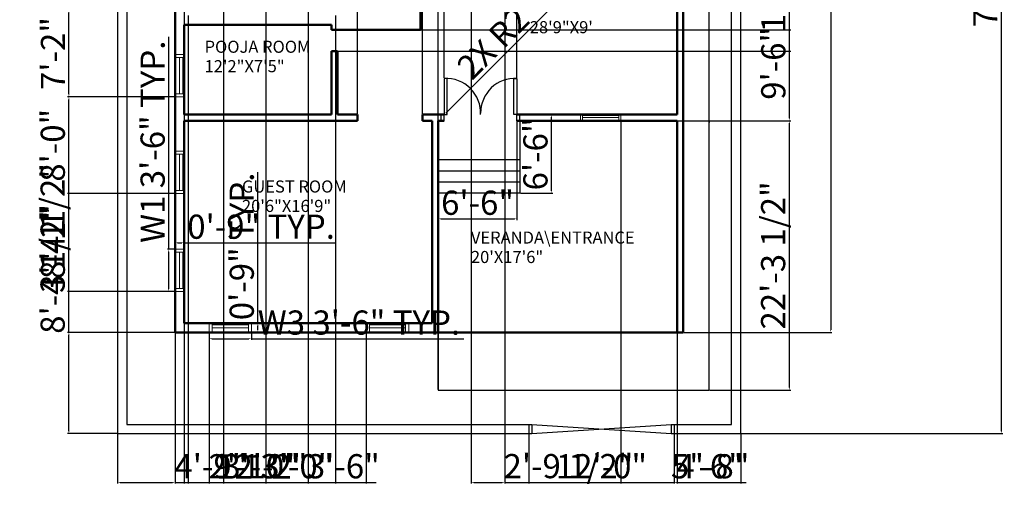
# Model space of a CAD drawing. Units: inches. Extents: x 2047 to 3023, y 479 to 1545.
# Tile 1 of 3: x 2047 to 3023, y 479 to 961. Entities that reach past the tile are written whole.
import ezdxf

# ---------------------------------------------------------------- set-up
doc = ezdxf.new("R2010")
doc.units = ezdxf.units.IN
for name, color, linetype, lineweight in [('A-ANNO-DIMS', 2, 'Continuous', 18), ('A-AREA-IDEN', 7, 'Continuous', 25), ('A-DOOR', 3, 'Continuous', 25), ('A-FLOR', 8, 'Continuous', 25), ('A-FLOR-STRS', 7, 'Continuous', 25), ('A-GLAZ', 4, 'Continuous', 18), ('A-WALL', 7, 'Continuous', 50), ('C-PROP', 8, 'Continuous', 30)]:
    doc.layers.add(name, color=color, linetype=linetype, lineweight=lineweight)
doc.styles.get("Standard").update_dxf_attribs({"font": 'arial.ttf'})
doc.dimstyles.new('ISO-25', dxfattribs={"dimtxt": 24, "dimasz": 2.5, "dimexe": 1.25, "dimexo": 0.625, "dimtad": 1, "dimdec": 1, "dimlunit": 3, "dimtxsty": 'Standard', "dimcen": 2.5, "dimadec": 0, "dimazin": 0, "dimtfac": 1, "dimtdec": 1, "dimtmove": 0, "dimatfit": 3, "dimfxl": 1, "dimarcsym": 0})

# ---------------------------------------------------------------- blocks, each defined once
blk = doc.blocks.new('*D3')
at = {"layer": 'A-ANNO-DIMS', "color": 0, "lineweight": -2, "transparency": 16777216}
for p, q in [((2762.53, 1447.48), (3021.8, 1447.48)), ((3020.55, 552.98), (3020.55, 1444.98)), ((2762.53, 550.48), (3021.8, 550.48))]:
    blk.add_line(p, q, dxfattribs=at)
at = {"layer": 'A-ANNO-DIMS', "color": 0, "transparency": 16777216}
for points in [[(3020.13, 1444.98), (3020.96, 1444.98), (3020.55, 1447.48)], [(3020.13, 552.98), (3020.96, 552.98), (3020.55, 550.48)]]:
    blk.add_solid(points, dxfattribs=at)
at = {"layer": 'Defpoints', "color": 0, "transparency": 16777216}
for p in [(2761.91, 1447.48), (3020.55, 1447.48), (2761.91, 550.48)]:
    blk.add_point(p, dxfattribs=at)
at = {"layer": 'A-ANNO-DIMS', "color": 0, "transparency": 16777216, "insert": (3007.67, 998.98), "char_height": 24, "attachment_point": 5, "rotation": 90}
blk.add_mtext('74\'-9"', dxfattribs=at)
blk = doc.blocks.new('*D6')
at = {"layer": 'A-ANNO-DIMS', "color": 0, "lineweight": -2, "transparency": 16777216}
for p, q in [((2705.53, 1346.98), (2852.44, 1346.98)), ((2851.19, 1344.48), (2851.19, 653.48)), ((2705.53, 650.98), (2852.44, 650.98))]:
    blk.add_line(p, q, dxfattribs=at)
at = {"layer": 'A-ANNO-DIMS', "color": 0, "transparency": 16777216}
for points in [[(2850.77, 1344.48), (2851.6, 1344.48), (2851.19, 1346.98)], [(2850.77, 653.48), (2851.6, 653.48), (2851.19, 650.98)]]:
    blk.add_solid(points, dxfattribs=at)
at = {"layer": 'Defpoints', "color": 0, "transparency": 16777216}
for p in [(2704.91, 1346.98), (2704.91, 650.98), (2851.19, 650.98)]:
    blk.add_point(p, dxfattribs=at)
at = {"layer": 'A-ANNO-DIMS', "color": 0, "transparency": 16777216, "insert": (2838.31, 998.98), "char_height": 24, "attachment_point": 5, "rotation": 90}
blk.add_mtext("58'", dxfattribs=at)
blk = doc.blocks.new('*D7')
at = {"layer": 'A-ANNO-DIMS', "color": 0, "lineweight": -2, "transparency": 16777216}
for p, q in [((2461.91, 788.36), (2461.91, 762.34)), ((2539.91, 788.36), (2539.91, 762.34)), ((2464.41, 763.59), (2537.41, 763.59))]:
    blk.add_line(p, q, dxfattribs=at)
at = {"layer": 'A-ANNO-DIMS', "color": 0, "transparency": 16777216}
for points in [[(2464.41, 764.01), (2464.41, 763.17), (2461.91, 763.59)], [(2537.41, 764.01), (2537.41, 763.17), (2539.91, 763.59)]]:
    blk.add_solid(points, dxfattribs=at)
at = {"layer": 'Defpoints', "color": 0, "transparency": 16777216}
for p in [(2461.91, 788.98), (2539.91, 788.98), (2539.91, 763.59)]:
    blk.add_point(p, dxfattribs=at)
at = {"layer": 'A-ANNO-DIMS', "color": 0, "transparency": 16777216, "insert": (2500.91, 776.47), "char_height": 24, "attachment_point": 5}
blk.add_mtext('6\'-6"', dxfattribs=at)
blk = doc.blocks.new('*D8')
at = {"layer": 'A-ANNO-DIMS', "color": 0, "lineweight": -2, "transparency": 16777216}
for p, q in [((2543.53, 866.98), (2575.53, 866.98)), ((2574.28, 791.48), (2574.28, 864.48)), ((2543.53, 788.98), (2575.53, 788.98))]:
    blk.add_line(p, q, dxfattribs=at)
at = {"layer": 'A-ANNO-DIMS', "color": 0, "transparency": 16777216}
for points in [[(2573.86, 864.48), (2574.7, 864.48), (2574.28, 866.98)], [(2573.86, 791.48), (2574.7, 791.48), (2574.28, 788.98)]]:
    blk.add_solid(points, dxfattribs=at)
at = {"layer": 'Defpoints', "color": 0, "transparency": 16777216}
for p in [(2542.91, 866.98), (2574.28, 866.98), (2542.91, 788.98)]:
    blk.add_point(p, dxfattribs=at)
at = {"layer": 'A-ANNO-DIMS', "color": 0, "transparency": 16777216, "insert": (2561.4, 827.98), "char_height": 24, "attachment_point": 5, "rotation": 90}
blk.add_mtext('6\'-6"', dxfattribs=at)
blk = doc.blocks.new('WIN-36IN-9IN-FRAME')
for p, q in [((9, 42), (0, 42)), ((9, 39), (0, 39)), ((0, 39), (0, 3)), ((4.5, 3), (4.5, 39)), ((7.5, 3), (7.5, 39)), ((9, 3), (9, 39)), ((0, 3), (9, 3)), ((0, 0), (9, 0))]:
    blk.add_line(p, q)
blk = doc.blocks.new('WIN-36IN-9IN-JAMBS')
for p, q in [((0, 9), (0, 0)), ((3, 9), (3, 0)), ((39, 7.5), (3, 7.5)), ((39, 4.5), (3, 4.5)), ((39, 0), (39, 9)), ((42, 0), (42, 9))]:
    blk.add_line(p, q)
blk = doc.blocks.new('WIN-36IN-6IN-FRAME')
for p, q in [((0, 6), (0, 0)), ((38, 6), (2, 6)), ((2, 6), (2, 0)), ((38, 5), (2, 5)), ((38, 3), (2, 3)), ((2, 0), (38, 0)), ((38, 0), (38, 6)), ((40, 0), (40, 6))]:
    blk.add_line(p, q)
blk = doc.blocks.new('*D14')
at = {"layer": 'A-ANNO-DIMS', "color": 0, "lineweight": -2, "transparency": 16777216}
for p, q in [((2194.61, 733.51), (2194.61, 944.14)), ((2200.28, 733.51), (2193.36, 733.51)), ((2194.61, 694.01), (2194.61, 731.01)), ((2200.28, 691.51), (2193.36, 691.51))]:
    blk.add_line(p, q, dxfattribs=at)
at = {"layer": 'A-ANNO-DIMS', "color": 0, "transparency": 16777216}
for points in [[(2194.19, 731.01), (2195.02, 731.01), (2194.61, 733.51)], [(2194.19, 694.01), (2195.02, 694.01), (2194.61, 691.51)]]:
    blk.add_solid(points, dxfattribs=at)
at = {"layer": 'Defpoints', "color": 0, "transparency": 16777216}
for p in [(2194.61, 733.51), (2200.91, 733.51), (2200.91, 691.51)]:
    blk.add_point(p, dxfattribs=at)
at = {"layer": 'A-ANNO-DIMS', "color": 0, "transparency": 16777216, "insert": (2181.72, 840.08), "char_height": 24, "attachment_point": 5, "rotation": 90}
blk.add_mtext('W1 3\'-6" TYP.', dxfattribs=at)
blk = doc.blocks.new('*D15')
at = {"layer": 'A-ANNO-DIMS', "color": 0, "lineweight": -2, "transparency": 16777216}
for p, q in [((2200.91, 734.14), (2200.91, 741.06)), ((2203.41, 739.81), (2207.41, 739.81)), ((2209.91, 734.14), (2209.91, 741.06)), ((2209.91, 739.81), (2359.95, 739.81))]:
    blk.add_line(p, q, dxfattribs=at)
at = {"layer": 'A-ANNO-DIMS', "color": 0, "transparency": 16777216}
for points in [[(2203.41, 740.23), (2203.41, 739.39), (2200.91, 739.81)], [(2207.41, 740.23), (2207.41, 739.39), (2209.91, 739.81)]]:
    blk.add_solid(points, dxfattribs=at)
at = {"layer": 'Defpoints', "color": 0, "transparency": 16777216}
for p in [(2200.91, 733.51), (2209.91, 739.81), (2209.91, 733.51)]:
    blk.add_point(p, dxfattribs=at)
at = {"layer": 'A-ANNO-DIMS', "color": 0, "transparency": 16777216, "insert": (2286.18, 752.69), "char_height": 24, "attachment_point": 5}
blk.add_mtext('0\'-9" TYP.', dxfattribs=at)
blk = doc.blocks.new('*D18')
at = {"layer": 'A-ANNO-DIMS', "color": 0, "lineweight": -2, "transparency": 16777216}
for p, q in [((2234.67, 650.36), (2234.67, 643.43)), ((2237.17, 644.68), (2274.17, 644.68)), ((2276.67, 650.36), (2276.67, 643.43)), ((2276.67, 644.68), (2487.3, 644.68))]:
    blk.add_line(p, q, dxfattribs=at)
at = {"layer": 'A-ANNO-DIMS', "color": 0, "transparency": 16777216}
for points in [[(2237.17, 645.1), (2237.17, 644.26), (2234.67, 644.68)], [(2274.17, 645.1), (2274.17, 644.26), (2276.67, 644.68)]]:
    blk.add_solid(points, dxfattribs=at)
at = {"layer": 'Defpoints', "color": 0, "transparency": 16777216}
for p in [(2234.67, 650.98), (2276.67, 650.98), (2276.67, 644.68)]:
    blk.add_point(p, dxfattribs=at)
at = {"layer": 'A-ANNO-DIMS', "color": 0, "transparency": 16777216, "insert": (2383.24, 657.57), "char_height": 24, "attachment_point": 5}
blk.add_mtext('W3 3\'-6" TYP.', dxfattribs=at)
blk = doc.blocks.new('*D19')
at = {"layer": 'A-ANNO-DIMS', "color": 0, "lineweight": -2, "transparency": 16777216}
for p, q in [((2282.97, 659.98), (2282.97, 810.02)), ((2277.3, 659.98), (2284.22, 659.98)), ((2282.97, 653.48), (2282.97, 657.48)), ((2277.3, 650.98), (2284.22, 650.98))]:
    blk.add_line(p, q, dxfattribs=at)
at = {"layer": 'A-ANNO-DIMS', "color": 0, "transparency": 16777216}
for points in [[(2282.56, 657.48), (2283.39, 657.48), (2282.97, 659.98)], [(2282.56, 653.48), (2283.39, 653.48), (2282.97, 650.98)]]:
    blk.add_solid(points, dxfattribs=at)
at = {"layer": 'Defpoints', "color": 0, "transparency": 16777216}
for p in [(2276.67, 659.98), (2282.97, 659.98), (2276.67, 650.98)]:
    blk.add_point(p, dxfattribs=at)
at = {"layer": 'A-ANNO-DIMS', "color": 0, "transparency": 16777216, "insert": (2270.09, 736.25), "char_height": 24, "attachment_point": 5, "rotation": 90}
blk.add_mtext('0\'-9" TYP.', dxfattribs=at)
blk = doc.blocks.new('*D20')
at = {"layer": 'A-ANNO-DIMS', "color": 0, "lineweight": -2, "transparency": 16777216}
for p, q in [((2200.91, 650.36), (2200.91, 500.88)), ((2143.91, 549.86), (2143.91, 500.88)), ((2146.41, 502.13), (2198.41, 502.13)), ((2200.91, 502.13), (2269.42, 502.13))]:
    blk.add_line(p, q, dxfattribs=at)
at = {"layer": 'A-ANNO-DIMS', "color": 0, "transparency": 16777216}
for points in [[(2146.41, 502.55), (2146.41, 501.71), (2143.91, 502.13)], [(2198.41, 502.55), (2198.41, 501.71), (2200.91, 502.13)]]:
    blk.add_solid(points, dxfattribs=at)
at = {"layer": 'Defpoints', "color": 0, "transparency": 16777216}
for p in [(2200.91, 650.98), (2143.91, 550.48), (2200.91, 502.13)]:
    blk.add_point(p, dxfattribs=at)
at = {"layer": 'A-ANNO-DIMS', "color": 0, "transparency": 16777216, "insert": (2236.41, 515.01), "char_height": 24, "attachment_point": 5}
blk.add_mtext('4\'-9"', dxfattribs=at)
blk = doc.blocks.new('*D21')
at = {"layer": 'A-ANNO-DIMS', "color": 0, "lineweight": -2, "transparency": 16777216}
for p, q in [((2095.56, 650.98), (2095.56, 774.48)), ((2200.28, 650.98), (2094.31, 650.98)), ((2095.56, 552.98), (2095.56, 648.48)), ((2143.28, 550.48), (2094.31, 550.48))]:
    blk.add_line(p, q, dxfattribs=at)
at = {"layer": 'A-ANNO-DIMS', "color": 0, "transparency": 16777216}
for points in [[(2095.14, 648.48), (2095.97, 648.48), (2095.56, 650.98)], [(2095.14, 552.98), (2095.97, 552.98), (2095.56, 550.48)]]:
    blk.add_solid(points, dxfattribs=at)
at = {"layer": 'Defpoints', "color": 0, "transparency": 16777216}
for p in [(2095.56, 650.98), (2200.91, 650.98), (2143.91, 550.48)]:
    blk.add_point(p, dxfattribs=at)
at = {"layer": 'A-ANNO-DIMS', "color": 0, "transparency": 16777216, "insert": (2082.52, 713.98), "char_height": 24, "attachment_point": 5, "rotation": 90}
blk.add_mtext('8\'-4 1/2"', dxfattribs=at)
blk = doc.blocks.new('*D22')
at = {"layer": 'A-ANNO-DIMS', "color": 0, "lineweight": -2, "transparency": 16777216}
for p, q in [((2551.81, 549.86), (2551.81, 500.88)), ((2695.81, 549.86), (2695.81, 500.88)), ((2554.31, 502.13), (2693.31, 502.13))]:
    blk.add_line(p, q, dxfattribs=at)
at = {"layer": 'A-ANNO-DIMS', "color": 0, "transparency": 16777216}
for points in [[(2554.31, 502.55), (2554.31, 501.71), (2551.81, 502.13)], [(2693.31, 502.55), (2693.31, 501.71), (2695.81, 502.13)]]:
    blk.add_solid(points, dxfattribs=at)
at = {"layer": 'Defpoints', "color": 0, "transparency": 16777216}
for p in [(2551.81, 550.48), (2695.81, 550.48), (2695.81, 502.13)]:
    blk.add_point(p, dxfattribs=at)
at = {"layer": 'A-ANNO-DIMS', "color": 0, "transparency": 16777216, "insert": (2623.81, 515.01), "char_height": 24, "attachment_point": 5}
blk.add_mtext('12\'-0"', dxfattribs=at)
blk = doc.blocks.new('*D23')
at = {"layer": 'A-ANNO-DIMS', "color": 0, "lineweight": -2, "transparency": 16777216}
for p, q in [((2695.81, 549.86), (2695.81, 500.88)), ((2761.91, 549.86), (2761.91, 500.88)), ((2698.31, 502.13), (2759.41, 502.13))]:
    blk.add_line(p, q, dxfattribs=at)
at = {"layer": 'A-ANNO-DIMS', "color": 0, "transparency": 16777216}
for points in [[(2698.31, 502.55), (2698.31, 501.71), (2695.81, 502.13)], [(2759.41, 502.55), (2759.41, 501.71), (2761.91, 502.13)]]:
    blk.add_solid(points, dxfattribs=at)
at = {"layer": 'Defpoints', "color": 0, "transparency": 16777216}
for p in [(2695.81, 550.48), (2761.91, 550.48), (2761.91, 502.13)]:
    blk.add_point(p, dxfattribs=at)
at = {"layer": 'A-ANNO-DIMS', "color": 0, "transparency": 16777216, "insert": (2728.86, 515.01), "char_height": 24, "attachment_point": 5}
blk.add_mtext('5\'-6"', dxfattribs=at)
blk = doc.blocks.new('*D24')
at = {"layer": 'A-ANNO-DIMS', "color": 0, "lineweight": -2, "transparency": 16777216}
for p, q in [((2461.91, 594.24), (2461.91, 1497.08)), ((2464.41, 1495.83), (2728.27, 1495.83)), ((2730.77, 594.24), (2730.77, 1497.08))]:
    blk.add_line(p, q, dxfattribs=at)
at = {"layer": 'A-ANNO-DIMS', "color": 0, "transparency": 16777216}
for points in [[(2464.41, 1496.25), (2464.41, 1495.41), (2461.91, 1495.83)], [(2728.27, 1496.25), (2728.27, 1495.41), (2730.77, 1495.83)]]:
    blk.add_solid(points, dxfattribs=at)
at = {"layer": 'Defpoints', "color": 0, "transparency": 16777216}
for p in [(2730.77, 1495.83), (2461.91, 593.62), (2730.77, 593.62)]:
    blk.add_point(p, dxfattribs=at)
at = {"layer": 'A-ANNO-DIMS', "color": 0, "transparency": 16777216, "insert": (2596.34, 1508.71), "char_height": 24, "attachment_point": 5}
blk.add_mtext('22\'-5"', dxfattribs=at)
blk = doc.blocks.new('*D25')
at = {"layer": 'A-ANNO-DIMS', "color": 0, "lineweight": -2, "transparency": 16777216}
for p, q in [((2731.39, 860.98), (2811.51, 860.98)), ((2810.26, 596.12), (2810.26, 858.48)), ((2731.39, 593.62), (2811.51, 593.62))]:
    blk.add_line(p, q, dxfattribs=at)
at = {"layer": 'A-ANNO-DIMS', "color": 0, "transparency": 16777216}
for points in [[(2809.84, 858.48), (2810.67, 858.48), (2810.26, 860.98)], [(2809.84, 596.12), (2810.67, 596.12), (2810.26, 593.62)]]:
    blk.add_solid(points, dxfattribs=at)
at = {"layer": 'Defpoints', "color": 0, "transparency": 16777216}
for p in [(2730.77, 860.98), (2810.26, 860.98), (2730.77, 593.62)]:
    blk.add_point(p, dxfattribs=at)
at = {"layer": 'A-ANNO-DIMS', "color": 0, "transparency": 16777216, "insert": (2797.22, 727.3), "char_height": 24, "attachment_point": 5, "rotation": 90}
blk.add_mtext('22\'-3 1/2"', dxfattribs=at)
blk = doc.blocks.new('*D26')
at = {"layer": 'A-ANNO-DIMS', "color": 0, "lineweight": -2, "transparency": 16777216}
for p, q in [((2095.56, 691.51), (2095.56, 814.97)), ((2200.28, 691.51), (2094.31, 691.51)), ((2095.56, 653.48), (2095.56, 689.01)), ((2200.28, 650.98), (2094.31, 650.98))]:
    blk.add_line(p, q, dxfattribs=at)
at = {"layer": 'A-ANNO-DIMS', "color": 0, "transparency": 16777216}
for points in [[(2095.14, 689.01), (2095.97, 689.01), (2095.56, 691.51)], [(2095.14, 653.48), (2095.97, 653.48), (2095.56, 650.98)]]:
    blk.add_solid(points, dxfattribs=at)
at = {"layer": 'Defpoints', "color": 0, "transparency": 16777216}
for p in [(2095.56, 691.51), (2200.91, 691.51), (2200.91, 650.98)]:
    blk.add_point(p, dxfattribs=at)
at = {"layer": 'A-ANNO-DIMS', "color": 0, "transparency": 16777216, "insert": (2082.52, 754.49), "char_height": 24, "attachment_point": 5, "rotation": 90}
blk.add_mtext('3\'-4 1/2"', dxfattribs=at)
blk = doc.blocks.new('*D27')
at = {"layer": 'A-ANNO-DIMS', "color": 0, "lineweight": -2, "transparency": 16777216}
for p, q in [((2200.28, 788.59), (2094.31, 788.59)), ((2095.56, 694.01), (2095.56, 786.09)), ((2200.28, 691.51), (2094.31, 691.51))]:
    blk.add_line(p, q, dxfattribs=at)
at = {"layer": 'A-ANNO-DIMS', "color": 0, "transparency": 16777216}
for points in [[(2095.14, 786.09), (2095.97, 786.09), (2095.56, 788.59)], [(2095.14, 694.01), (2095.97, 694.01), (2095.56, 691.51)]]:
    blk.add_solid(points, dxfattribs=at)
at = {"layer": 'Defpoints', "color": 0, "transparency": 16777216}
for p in [(2095.56, 788.59), (2200.91, 788.59), (2200.91, 691.51)]:
    blk.add_point(p, dxfattribs=at)
at = {"layer": 'A-ANNO-DIMS', "color": 0, "transparency": 16777216, "insert": (2082.68, 740.05), "char_height": 24, "attachment_point": 5, "rotation": 90}
blk.add_mtext('8\'-1"', dxfattribs=at)
blk = doc.blocks.new('*D28')
at = {"layer": 'A-ANNO-DIMS', "color": 0, "lineweight": -2, "transparency": 16777216}
for p, q in [((2200.28, 884.62), (2094.31, 884.62)), ((2095.56, 791.09), (2095.56, 882.12)), ((2200.28, 788.59), (2094.31, 788.59))]:
    blk.add_line(p, q, dxfattribs=at)
at = {"layer": 'A-ANNO-DIMS', "color": 0, "transparency": 16777216}
for points in [[(2095.14, 882.12), (2095.97, 882.12), (2095.56, 884.62)], [(2095.14, 791.09), (2095.97, 791.09), (2095.56, 788.59)]]:
    blk.add_solid(points, dxfattribs=at)
at = {"layer": 'Defpoints', "color": 0, "transparency": 16777216}
for p in [(2095.56, 884.62), (2200.91, 884.62), (2200.91, 788.59)]:
    blk.add_point(p, dxfattribs=at)
at = {"layer": 'A-ANNO-DIMS', "color": 0, "transparency": 16777216, "insert": (2082.68, 836.61), "char_height": 24, "attachment_point": 5, "rotation": 90}
blk.add_mtext('8\'-0"', dxfattribs=at)
blk = doc.blocks.new('*D29')
at = {"layer": 'A-ANNO-DIMS', "color": 0, "lineweight": -2, "transparency": 16777216}
for p, q in [((2200.28, 970.66), (2094.31, 970.66)), ((2095.56, 887.12), (2095.56, 968.16)), ((2200.28, 884.62), (2094.31, 884.62))]:
    blk.add_line(p, q, dxfattribs=at)
at = {"layer": 'A-ANNO-DIMS', "color": 0, "transparency": 16777216}
for points in [[(2095.14, 968.16), (2095.97, 968.16), (2095.56, 970.66)], [(2095.14, 887.12), (2095.97, 887.12), (2095.56, 884.62)]]:
    blk.add_solid(points, dxfattribs=at)
at = {"layer": 'Defpoints', "color": 0, "transparency": 16777216}
for p in [(2095.56, 970.66), (2200.91, 970.66), (2200.91, 884.62)]:
    blk.add_point(p, dxfattribs=at)
at = {"layer": 'A-ANNO-DIMS', "color": 0, "transparency": 16777216, "insert": (2082.88, 927.64), "char_height": 24, "attachment_point": 5, "rotation": 90}
blk.add_mtext('7\'-2"', dxfattribs=at)
blk = doc.blocks.new('*D32')
at = {"layer": 'A-ANNO-DIMS', "color": 0, "lineweight": -2, "transparency": 16777216}
for p, q in [((2705.53, 974.8), (2811.51, 974.8)), ((2810.26, 863.48), (2810.26, 972.3)), ((2699.53, 860.98), (2811.51, 860.98))]:
    blk.add_line(p, q, dxfattribs=at)
at = {"layer": 'A-ANNO-DIMS', "color": 0, "transparency": 16777216}
for points in [[(2809.84, 972.3), (2810.67, 972.3), (2810.26, 974.8)], [(2809.84, 863.48), (2810.67, 863.48), (2810.26, 860.98)]]:
    blk.add_solid(points, dxfattribs=at)
at = {"layer": 'Defpoints', "color": 0, "transparency": 16777216}
for p in [(2704.91, 974.8), (2810.26, 974.8), (2698.91, 860.98)]:
    blk.add_point(p, dxfattribs=at)
at = {"layer": 'A-ANNO-DIMS', "color": 0, "transparency": 16777216, "insert": (2797.38, 917.89), "char_height": 24, "attachment_point": 5, "rotation": 90}
blk.add_mtext('9\'-6"', dxfattribs=at)
blk = doc.blocks.new('*D35')
at = {"layer": 'A-ANNO-DIMS', "color": 0, "lineweight": -2, "transparency": 16777216}
for p, q in [((2200.91, 650.36), (2200.91, 500.88)), ((2234.67, 650.36), (2234.67, 500.88)), ((2203.41, 502.13), (2232.17, 502.13)), ((2234.67, 502.13), (2321.28, 502.13))]:
    blk.add_line(p, q, dxfattribs=at)
at = {"layer": 'A-ANNO-DIMS', "color": 0, "transparency": 16777216}
for points in [[(2203.41, 502.55), (2203.41, 501.71), (2200.91, 502.13)], [(2232.17, 502.55), (2232.17, 501.71), (2234.67, 502.13)]]:
    blk.add_solid(points, dxfattribs=at)
at = {"layer": 'Defpoints', "color": 0, "transparency": 16777216}
for p in [(2200.91, 650.98), (2234.67, 650.98), (2234.67, 502.13)]:
    blk.add_point(p, dxfattribs=at)
at = {"layer": 'A-ANNO-DIMS', "color": 0, "transparency": 16777216, "insert": (2279.23, 515.01), "char_height": 24, "attachment_point": 5}
blk.add_mtext('2\'-10"', dxfattribs=at)
blk = doc.blocks.new('*D36')
at = {"layer": 'A-ANNO-DIMS', "color": 0, "lineweight": -2, "transparency": 16777216}
for p, q in [((2234.67, 650.36), (2234.67, 500.88)), ((2390.57, 650.36), (2390.57, 500.88)), ((2237.17, 502.13), (2388.07, 502.13))]:
    blk.add_line(p, q, dxfattribs=at)
at = {"layer": 'A-ANNO-DIMS', "color": 0, "transparency": 16777216}
for points in [[(2237.17, 502.55), (2237.17, 501.71), (2234.67, 502.13)], [(2388.07, 502.55), (2388.07, 501.71), (2390.57, 502.13)]]:
    blk.add_solid(points, dxfattribs=at)
at = {"layer": 'Defpoints', "color": 0, "transparency": 16777216}
for p in [(2234.67, 650.98), (2390.57, 650.98), (2390.57, 502.13)]:
    blk.add_point(p, dxfattribs=at)
at = {"layer": 'A-ANNO-DIMS', "color": 0, "transparency": 16777216, "insert": (2312.62, 515.02), "char_height": 24, "attachment_point": 5}
blk.add_mtext('13\'-0"', dxfattribs=at)
blk = doc.blocks.new('*D37')
at = {"layer": 'A-ANNO-DIMS', "color": 0, "lineweight": -2, "transparency": 16777216}
for p, q in [((2290.91, 1340.36), (2290.91, 500.88)), ((2332.76, 1340.36), (2332.76, 500.88)), ((2293.41, 502.13), (2330.26, 502.13)), ((2332.76, 502.13), (2400.29, 502.13))]:
    blk.add_line(p, q, dxfattribs=at)
at = {"layer": 'A-ANNO-DIMS', "color": 0, "transparency": 16777216}
for points in [[(2293.41, 502.55), (2293.41, 501.71), (2290.91, 502.13)], [(2330.26, 502.55), (2330.26, 501.71), (2332.76, 502.13)]]:
    blk.add_solid(points, dxfattribs=at)
at = {"layer": 'Defpoints', "color": 0, "transparency": 16777216}
for p in [(2290.91, 1340.98), (2332.76, 1340.98), (2332.76, 502.13)]:
    blk.add_point(p, dxfattribs=at)
at = {"layer": 'A-ANNO-DIMS', "color": 0, "transparency": 16777216, "insert": (2367.78, 515.02), "char_height": 24, "attachment_point": 5}
blk.add_mtext('3\'-6"', dxfattribs=at)
blk = doc.blocks.new('*D38')
at = {"layer": 'A-ANNO-DIMS', "color": 0, "lineweight": -2, "transparency": 16777216}
for p, q in [((2494.55, 1340.36), (2494.55, 500.88)), ((2527.91, 1340.36), (2527.91, 500.88)), ((2497.05, 502.13), (2525.41, 502.13)), ((2527.91, 502.13), (2651.79, 502.13))]:
    blk.add_line(p, q, dxfattribs=at)
at = {"layer": 'A-ANNO-DIMS', "color": 0, "transparency": 16777216}
for points in [[(2497.05, 502.55), (2497.05, 501.71), (2494.55, 502.13)], [(2525.41, 502.55), (2525.41, 501.71), (2527.91, 502.13)]]:
    blk.add_solid(points, dxfattribs=at)
at = {"layer": 'Defpoints', "color": 0, "transparency": 16777216}
for p in [(2494.55, 1340.98), (2527.91, 1340.98), (2527.91, 502.13)]:
    blk.add_point(p, dxfattribs=at)
at = {"layer": 'A-ANNO-DIMS', "color": 0, "transparency": 16777216, "insert": (2591.1, 515.16), "char_height": 24, "attachment_point": 5}
blk.add_mtext('2\'-9 1/2"', dxfattribs=at)
blk = doc.blocks.new('*D40')
at = {"layer": 'A-ANNO-DIMS', "color": 0, "lineweight": -2, "transparency": 16777216}
for p, q in [((2643.03, 860.36), (2643.03, 500.88)), ((2698.91, 860.36), (2698.91, 500.88)), ((2645.53, 502.13), (2696.41, 502.13)), ((2698.91, 502.13), (2767.42, 502.13))]:
    blk.add_line(p, q, dxfattribs=at)
at = {"layer": 'A-ANNO-DIMS', "color": 0, "transparency": 16777216}
for points in [[(2645.53, 502.55), (2645.53, 501.71), (2643.03, 502.13)], [(2696.41, 502.55), (2696.41, 501.71), (2698.91, 502.13)]]:
    blk.add_solid(points, dxfattribs=at)
at = {"layer": 'Defpoints', "color": 0, "transparency": 16777216}
for p in [(2643.03, 860.98), (2698.91, 860.98), (2698.91, 502.13)]:
    blk.add_point(p, dxfattribs=at)
at = {"layer": 'A-ANNO-DIMS', "color": 0, "transparency": 16777216, "insert": (2734.41, 515.01), "char_height": 24, "attachment_point": 5}
blk.add_mtext('4\'-8"', dxfattribs=at)
blk = doc.blocks.new('*D41')
at = {"layer": 'A-ANNO-DIMS', "color": 0, "lineweight": -2, "transparency": 16777216}
for p, q in [((2381.88, 867.61), (2381.88, 1497.08)), ((2384.38, 1495.83), (2443.66, 1495.83)), ((2446.16, 867.61), (2446.16, 1497.08)), ((2446.16, 1495.83), (2569.64, 1495.83))]:
    blk.add_line(p, q, dxfattribs=at)
at = {"layer": 'A-ANNO-DIMS', "color": 0, "transparency": 16777216}
for points in [[(2384.38, 1496.25), (2384.38, 1495.41), (2381.88, 1495.83)], [(2443.66, 1496.25), (2443.66, 1495.41), (2446.16, 1495.83)]]:
    blk.add_solid(points, dxfattribs=at)
at = {"layer": 'Defpoints', "color": 0, "transparency": 16777216}
for p in [(2446.16, 1495.83), (2381.88, 866.98), (2446.16, 866.98)]:
    blk.add_point(p, dxfattribs=at)
at = {"layer": 'A-ANNO-DIMS', "color": 0, "transparency": 16777216, "insert": (2509.15, 1508.86), "char_height": 24, "attachment_point": 5}
blk.add_mtext('5\'-4 1/2"', dxfattribs=at)
blk = doc.blocks.new('*D42')
at = {"layer": 'A-ANNO-DIMS', "color": 0, "lineweight": -2, "transparency": 16777216}
for p, q in [((2810.26, 950.97), (2810.26, 1016.25)), ((2362.53, 950.97), (2811.51, 950.97)), ((2810.26, 932.42), (2810.26, 948.47)), ((2362.53, 929.92), (2811.51, 929.92))]:
    blk.add_line(p, q, dxfattribs=at)
at = {"layer": 'A-ANNO-DIMS', "color": 0, "transparency": 16777216}
for points in [[(2809.84, 948.47), (2810.67, 948.47), (2810.26, 950.97)], [(2809.84, 932.42), (2810.67, 932.42), (2810.26, 929.92)]]:
    blk.add_solid(points, dxfattribs=at)
at = {"layer": 'Defpoints', "color": 0, "transparency": 16777216}
for p in [(2361.91, 950.97), (2810.26, 950.97), (2361.91, 929.92)]:
    blk.add_point(p, dxfattribs=at)
at = {"layer": 'A-ANNO-DIMS', "color": 0, "transparency": 16777216, "insert": (2797.38, 984.86), "char_height": 24, "attachment_point": 5, "rotation": 90}
blk.add_mtext('1\'-9"', dxfattribs=at)
blk = doc.blocks.new('*D43')
at = {"layer": 'A-ANNO-DIMS', "color": 0, "lineweight": -2, "transparency": 16777216}
for p, q in [((2213.91, 965.36), (2213.91, 500.88)), ((2359.91, 965.36), (2359.91, 500.88)), ((2216.41, 502.13), (2357.41, 502.13))]:
    blk.add_line(p, q, dxfattribs=at)
at = {"layer": 'A-ANNO-DIMS', "color": 0, "transparency": 16777216}
for points in [[(2216.41, 502.55), (2216.41, 501.71), (2213.91, 502.13)], [(2357.41, 502.55), (2357.41, 501.71), (2359.91, 502.13)]]:
    blk.add_solid(points, dxfattribs=at)
at = {"layer": 'Defpoints', "color": 0, "transparency": 16777216}
for p in [(2213.91, 965.98), (2359.91, 965.98), (2359.91, 502.13)]:
    blk.add_point(p, dxfattribs=at)
at = {"layer": 'A-ANNO-DIMS', "color": 0, "transparency": 16777216, "insert": (2286.91, 514.8), "char_height": 24, "attachment_point": 5}
blk.add_mtext('12\'-2"', dxfattribs=at)
blk = doc.blocks.new('*D51')
at = {"layer": 'A-ANNO-DIMS', "color": 0, "lineweight": -2, "transparency": 16777216}
for p, q in [((2467.91, 903.61), (2467.91, 1497.08)), ((2470.41, 1495.83), (2537.41, 1495.83)), ((2539.91, 903.61), (2539.91, 1497.08))]:
    blk.add_line(p, q, dxfattribs=at)
at = {"layer": 'A-ANNO-DIMS', "color": 0, "transparency": 16777216}
for points in [[(2470.41, 1496.25), (2470.41, 1495.41), (2467.91, 1495.83)], [(2537.41, 1496.25), (2537.41, 1495.41), (2539.91, 1495.83)]]:
    blk.add_solid(points, dxfattribs=at)
at = {"layer": 'Defpoints', "color": 0, "transparency": 16777216}
for p in [(2539.91, 1495.83), (2467.91, 902.98), (2539.91, 902.98)]:
    blk.add_point(p, dxfattribs=at)
at = {"layer": 'A-ANNO-DIMS', "color": 0, "transparency": 16777216, "insert": (2503.91, 1508.71), "char_height": 24, "attachment_point": 5}
blk.add_mtext('6\'-0"', dxfattribs=at)
blk = doc.blocks.new('*D53')
at = {"layer": 'A-ANNO-DIMS', "color": 0, "lineweight": -2, "transparency": 16777216}
for p, q in [((2209.91, 1346.36), (2209.91, 500.88)), ((2248.87, 1346.36), (2248.87, 500.88)), ((2212.41, 502.13), (2246.37, 502.13)), ((2248.87, 502.13), (2316.4, 502.13))]:
    blk.add_line(p, q, dxfattribs=at)
at = {"layer": 'A-ANNO-DIMS', "color": 0, "transparency": 16777216}
for points in [[(2212.41, 502.55), (2212.41, 501.71), (2209.91, 502.13)], [(2246.37, 502.55), (2246.37, 501.71), (2248.87, 502.13)]]:
    blk.add_solid(points, dxfattribs=at)
at = {"layer": 'Defpoints', "color": 0, "transparency": 16777216}
for p in [(2209.91, 1346.98), (2248.87, 1346.98), (2248.87, 502.13)]:
    blk.add_point(p, dxfattribs=at)
at = {"layer": 'A-ANNO-DIMS', "color": 0, "transparency": 16777216, "insert": (2283.89, 515.02), "char_height": 24, "attachment_point": 5}
blk.add_mtext('3\'-3"', dxfattribs=at)
blk = doc.blocks.new('*D54')
at = {"layer": 'A-ANNO-DIMS', "color": 0, "lineweight": -2, "transparency": 16777216}
for p, q in [((2649.08, 1048.15), (2495.59, 894.67)), ((2469.41, 868.48), (2493.83, 892.9))]:
    blk.add_line(p, q, dxfattribs=at)
at = {"layer": 'A-ANNO-DIMS', "color": 0, "transparency": 16777216}
blk.add_solid([(2495.3, 894.96), (2495.89, 894.37), (2493.83, 892.9)], dxfattribs=at)
at = {"layer": 'Defpoints', "color": 0, "transparency": 16777216}
for p in [(2493.83, 892.9), (2469.41, 868.48)]:
    blk.add_point(p, dxfattribs=at)
at = {"layer": 'A-ANNO-DIMS', "color": 0, "transparency": 16777216, "insert": (2564.01, 981.51), "char_height": 24, "attachment_point": 5, "rotation": 44.99969}
blk.add_mtext('2X R2\'-10 1/2"', dxfattribs=at)

msp = doc.modelspace()

# ---------------------------------------------------------------- linework, layer by layer
at = {"layer": 'A-DOOR'}
for p, q in [((2464.91, 860.98), (2464.91, 866.98)), ((2467.91, 860.98), (2467.91, 866.98)), ((2539.91, 860.98), (2539.91, 866.98)), ((2542.91, 860.98), (2542.91, 866.98))]:
    msp.add_line(p, q, dxfattribs=at)
for points in [[(2467.91, 866.98), (2470.91, 866.98), (2470.91, 902.98), (2467.91, 902.98)], [(2539.91, 866.98), (2536.91, 866.98), (2536.91, 902.98), (2539.91, 902.98)]]:
    msp.add_lwpolyline(points, close=True, dxfattribs=at)
for centre, radius, start, end in [((2469.41, 868.48), 34.53, 357.51045, 92.48955), ((2538.41, 868.54), 34.47, 87.50574, 180.09411)]:
    msp.add_arc(centre, radius, start, end, dxfattribs=at)
at = {"layer": 'A-FLOR'}
for p, q in [((2698.91, 860.98), (2730.77, 860.98)), ((2730.77, 860.98), (2730.77, 859.02)), ((2730.77, 593.62), (2730.77, 860.27)), ((2461.91, 650.98), (2461.91, 593.62)), ((2461.91, 593.62), (2730.77, 593.62))]:
    msp.add_line(p, q, dxfattribs=at)
at = {"layer": 'A-FLOR-STRS'}
for p, q in [((2539.91, 860.98), (2539.91, 788.98)), ((2542.91, 860.98), (2542.91, 788.98)), ((2542.91, 821.98), (2461.91, 821.98)), ((2542.91, 810.98), (2461.91, 810.98)), ((2542.91, 799.98), (2461.91, 799.98)), ((2542.91, 788.98), (2461.91, 788.98))]:
    msp.add_line(p, q, dxfattribs=at)
at = {"layer": 'A-WALL'}
for p, q in [((2200.91, 1346.98), (2200.91, 650.98)), ((2704.91, 650.98), (2704.91, 1346.98)), ((2698.91, 866.98), (2698.91, 1265.98)), ((2444.25, 950.97), (2444.25, 1035.32)), ((2209.91, 955.98), (2355.91, 955.98)), ((2209.91, 955.98), (2209.91, 866.98)), ((2355.91, 955.98), (2355.91, 950.97)), ((2355.91, 950.97), (2361.91, 950.97)), ((2361.91, 950.97), (2444.25, 950.97)), ((2355.91, 929.92), (2361.91, 929.92)), ((2355.91, 929.92), (2355.91, 866.98)), ((2361.91, 929.92), (2361.91, 866.98)), ((2209.91, 866.98), (2355.91, 866.98)), ((2209.91, 860.98), (2355.91, 860.98)), ((2209.91, 860.98), (2209.91, 659.98)), ((2355.91, 860.98), (2381.88, 860.98)), ((2361.91, 866.98), (2381.88, 866.98)), ((2381.88, 860.98), (2381.88, 866.98)), ((2446.16, 860.98), (2446.16, 866.98)), ((2446.16, 866.98), (2467.91, 866.98)), ((2446.16, 860.98), (2455.91, 860.98)), ((2455.91, 860.98), (2455.91, 659.98)), ((2461.91, 860.98), (2461.91, 650.98)), ((2461.91, 860.98), (2467.91, 860.98)), ((2539.91, 866.98), (2698.91, 866.98)), ((2539.91, 860.98), (2698.91, 860.98)), ((2698.91, 650.98), (2698.91, 860.98)), ((2209.91, 659.98), (2455.91, 659.98)), ((2200.91, 650.98), (2704.91, 650.98))]:
    msp.add_line(p, q, dxfattribs=at)
at = {"layer": 'C-PROP'}
for p, q in [((2551.81, 559.48), (2551.81, 550.48)), ((2554.81, 559.48), (2554.81, 550.48)), ((2554.81, 559.48), (2692.81, 550.48)), ((2554.81, 550.48), (2692.81, 559.48)), ((2692.81, 559.48), (2692.81, 550.48)), ((2695.81, 559.48), (2695.81, 550.48))]:
    msp.add_line(p, q, dxfattribs=at)
for points in [[(2692.81, 550.48), (2761.91, 550.48), (2761.91, 1447.48), (2143.91, 1447.48), (2143.91, 550.48), (2554.81, 550.48)], [(2692.81, 559.48), (2752.91, 559.48), (2752.91, 1438.48), (2152.91, 1438.48), (2152.91, 559.48), (2554.81, 559.48)]]:
    msp.add_lwpolyline(points, dxfattribs=at)

# ---------------------------------------------------------------- block references
at = {"layer": 'A-GLAZ'}
for name, p in [('WIN-36IN-9IN-FRAME', (2200.91, 884.62)), ('WIN-36IN-6IN-FRAME', (2603.03, 860.98)), ('WIN-36IN-9IN-FRAME', (2200.91, 788.59)), ('WIN-36IN-9IN-FRAME', (2200.91, 691.51)), ('WIN-36IN-9IN-JAMBS', (2234.67, 650.98)), ('WIN-36IN-9IN-JAMBS', (2390.57, 650.98))]:
    msp.add_blockref(name, p, dxfattribs=at)

# ---------------------------------------------------------------- texts
at = {"layer": 'A-AREA-IDEN'}
for s, p in [('28\'9"X9\'', (2552.73, 947.73)), ('POOJA ROOM', (2230.13, 928.31)), ('12\'2"X7\'5"', (2230.13, 909.03)), ('GUEST ROOM', (2267.23, 789.67)), ('20\'6"X16\'9"', (2267.23, 770.4)), ('VERANDA\\ENTRANCE', (2494.35, 739.01)), ('20\'X17\'6"', (2494.35, 719.74))]:
    msp.add_text(s, height=12, dxfattribs=at).set_placement(p)

# ---------------------------------------------------------------- dimensions: what is measured, and where the dimension line sits
at = {"layer": 'A-ANNO-DIMS'}
for base, p1, p2, override, picture, middle in [((2446.16, 1495.83), (2381.88, 866.98), (2446.16, 866.98), {"dimdec": 1, "dimlfac": 1, "dimrnd": 0, "dimzin": 1, "dimdsep": 46, "dimlunit": 4, "dimfrac": 2}, '*D41', (2509.15, 1508.86)), ((2730.77, 1495.83), (2461.91, 593.62), (2730.77, 593.62), {"dimdec": 1, "dimlfac": 1, "dimrnd": 0, "dimzin": 1, "dimdsep": 46, "dimlunit": 4, "dimfrac": 2}, '*D24', (2596.34, 1508.71)), ((2539.91, 1495.83), (2467.91, 902.98), (2539.91, 902.98), {"dimdec": 1, "dimlfac": 1, "dimrnd": 0, "dimzin": 1, "dimdsep": 46, "dimlunit": 4, "dimfrac": 2}, '*D51', (2503.91, 1508.71)), ((2248.87, 502.13), (2209.91, 1346.98), (2248.87, 1346.98), {"dimdec": 1, "dimlfac": 1, "dimrnd": 0, "dimzin": 1, "dimdsep": 46, "dimlunit": 4, "dimfrac": 2}, '*D53', (2283.89, 515.02)), ((2332.7623, 502.1302), (2290.908, 1340.9802), (2332.7623, 1340.9802), {"dimdec": 1, "dimlfac": 1, "dimrnd": 0, "dimzin": 1, "dimdsep": 46, "dimlunit": 4, "dimfrac": 2}, '*D37', (2367.7782, 515.0172)), ((2527.91, 502.13), (2494.55, 1340.98), (2527.91, 1340.98), {"dimdec": 1, "dimlfac": 1, "dimrnd": 0, "dimzin": 1, "dimdsep": 46, "dimlunit": 4, "dimfrac": 2}, '*D38', (2591.1, 515.16)), ((2359.91, 502.13), (2213.91, 965.98), (2359.91, 965.98), {"dimdec": 1, "dimlfac": 1, "dimrnd": 0, "dimzin": 1, "dimdsep": 46, "dimlunit": 4, "dimfrac": 2}, '*D43', (2286.91, 514.8)), ((2698.91, 502.13), (2643.03, 860.98), (2698.91, 860.98), {"dimdec": 1, "dimlfac": 1, "dimrnd": 0, "dimzin": 1, "dimdsep": 46, "dimlunit": 4, "dimfrac": 2}, '*D40', (2734.41, 515.01)), ((2539.91, 763.59), (2461.91, 788.98), (2539.91, 788.98), {"dimclrd": 0, "dimclre": 0, "dimclrt": 0}, '*D7', (2500.91, 776.47)), ((2200.91, 502.13), (2143.91, 550.48), (2200.91, 650.98), {"dimdec": 1, "dimlfac": 1, "dimrnd": 0, "dimzin": 1, "dimdsep": 46, "dimlunit": 4, "dimfrac": 2}, '*D20', (2236.41, 515.01)), ((2234.67, 502.13), (2200.91, 650.98), (2234.67, 650.98), {"dimdec": 1, "dimlfac": 1, "dimrnd": 0, "dimzin": 1, "dimdsep": 46, "dimlunit": 4, "dimfrac": 2}, '*D35', (2279.23, 515.01)), ((2390.57, 502.13), (2234.67, 650.98), (2390.57, 650.98), {"dimdec": 1, "dimlfac": 1, "dimrnd": 0, "dimzin": 1, "dimdsep": 46, "dimlunit": 4, "dimfrac": 2}, '*D36', (2312.62, 515.02)), ((2695.81, 502.13), (2551.81, 550.48), (2695.81, 550.48), {"dimdec": 1, "dimlfac": 1, "dimrnd": 0, "dimzin": 1, "dimdsep": 46, "dimlunit": 4, "dimfrac": 2}, '*D22', (2623.81, 515.01)), ((2761.91, 502.13), (2695.81, 550.48), (2761.91, 550.48), {"dimdec": 1, "dimlfac": 1, "dimrnd": 0, "dimzin": 1, "dimdsep": 46, "dimlunit": 4, "dimfrac": 2}, '*D23', (2728.86, 515.01))]:
    dim = msp.add_linear_dim(base=base, p1=p1, p2=p2, dimstyle='ISO-25', override=override, dxfattribs=at)
    dim.commit()
    dim.dimension.update_dxf_attribs({"geometry": picture, "text_midpoint": middle})
for base, p1, p2, override, picture, middle in [((3020.55, 1447.48), (2761.91, 550.48), (2761.91, 1447.48), {"dimclrd": 0, "dimclre": 0, "dimclrt": 0}, '*D3', (3007.67, 998.98)), ((2851.19, 650.98), (2704.91, 1346.98), (2704.91, 650.98), {"dimclrd": 0, "dimclre": 0, "dimclrt": 0}, '*D6', (2838.31, 998.98)), ((2810.258, 950.966), (2361.908, 929.9219), (2361.908, 950.966), {"dimdec": 1, "dimlfac": 1, "dimrnd": 0, "dimzin": 1, "dimdsep": 46, "dimlunit": 4, "dimfrac": 2}, '*D42', (2797.3792, 984.8604)), ((2095.56, 970.66), (2200.91, 884.62), (2200.91, 970.66), {"dimdec": 1, "dimlfac": 1, "dimrnd": 0, "dimzin": 1, "dimdsep": 46, "dimlunit": 4, "dimfrac": 2}, '*D29', (2082.88, 927.64)), ((2810.26, 974.8), (2698.91, 860.98), (2704.91, 974.8), {"dimdec": 1, "dimlfac": 1, "dimrnd": 0, "dimzin": 1, "dimdsep": 46, "dimlunit": 4, "dimfrac": 2}, '*D32', (2797.38, 917.89)), ((2095.56, 884.62), (2200.91, 788.59), (2200.91, 884.62), {"dimdec": 1, "dimlfac": 1, "dimrnd": 0, "dimzin": 1, "dimdsep": 46, "dimlunit": 4, "dimfrac": 2}, '*D28', (2082.68, 836.61)), ((2574.28, 866.98), (2542.91, 788.98), (2542.91, 866.98), {"dimclrd": 0, "dimclre": 0, "dimclrt": 0}, '*D8', (2561.4, 827.98)), ((2810.26, 860.98), (2730.77, 593.62), (2730.77, 860.98), {"dimdec": 1, "dimlfac": 1, "dimrnd": 0, "dimzin": 1, "dimdsep": 46, "dimlunit": 4, "dimfrac": 2}, '*D25', (2797.22, 727.3)), ((2095.56, 691.51), (2200.91, 650.98), (2200.91, 691.51), {"dimdec": 1, "dimlfac": 1, "dimrnd": 0, "dimzin": 1, "dimdsep": 46, "dimlunit": 4, "dimfrac": 2}, '*D26', (2082.52, 754.49)), ((2095.56, 788.59), (2200.91, 691.51), (2200.91, 788.59), {"dimdec": 1, "dimlfac": 1, "dimrnd": 0, "dimzin": 1, "dimdsep": 46, "dimlunit": 4, "dimfrac": 2}, '*D27', (2082.68, 740.05)), ((2095.56, 650.98), (2143.91, 550.48), (2200.91, 650.98), {"dimdec": 1, "dimlfac": 1, "dimrnd": 0, "dimzin": 1, "dimdsep": 46, "dimlunit": 4, "dimfrac": 2}, '*D21', (2082.52, 713.98))]:
    dim = msp.add_linear_dim(base=base, p1=p1, p2=p2, angle=90, dimstyle='ISO-25', override=override, dxfattribs=at)
    dim.commit()
    dim.dimension.update_dxf_attribs({"geometry": picture, "text_midpoint": middle})
dim = msp.add_radius_dim(center=(2469.41, 868.48), mpoint=(2493.83, 892.9), text='2X <>', dimstyle='ISO-25', override={"dimdec": 1, "dimlfac": 1, "dimrnd": 0, "dimzin": 1, "dimdsep": 46, "dimlunit": 4, "dimfrac": 2}, dxfattribs=at)
dim.commit()
dim.dimension.update_dxf_attribs({"geometry": '*D54', "text_midpoint": (2564.01, 981.51)})
for base, p1, p2, text, picture, middle in [((2194.61, 733.51), (2200.91, 691.51), (2200.91, 733.51), 'W1 <> TYP.', '*D14', (2181.72, 840.08)), ((2282.97, 659.98), (2276.67, 650.98), (2276.67, 659.98), '<> TYP.', '*D19', (2270.09, 736.25))]:
    dim = msp.add_linear_dim(base=base, p1=p1, p2=p2, angle=90, text=text, dimstyle='ISO-25', override={"dimdec": 1, "dimlfac": 1, "dimrnd": 0, "dimzin": 1, "dimdsep": 46, "dimlunit": 4, "dimfrac": 2}, dxfattribs=at)
    dim.commit()
    dim.dimension.update_dxf_attribs({"geometry": picture, "text_midpoint": middle})
for base, p1, p2, text, picture, middle in [((2209.91, 739.81), (2200.91, 733.51), (2209.91, 733.51), '<> TYP.', '*D15', (2286.18, 752.69)), ((2276.67, 644.68), (2234.67, 650.98), (2276.67, 650.98), 'W3 <> TYP.', '*D18', (2383.24, 657.57))]:
    dim = msp.add_linear_dim(base=base, p1=p1, p2=p2, text=text, dimstyle='ISO-25', override={"dimdec": 1, "dimlfac": 1, "dimrnd": 0, "dimzin": 1, "dimdsep": 46, "dimlunit": 4, "dimfrac": 2}, dxfattribs=at)
    dim.commit()
    dim.dimension.update_dxf_attribs({"geometry": picture, "text_midpoint": middle})

doc.saveas('drawing.dxf')
